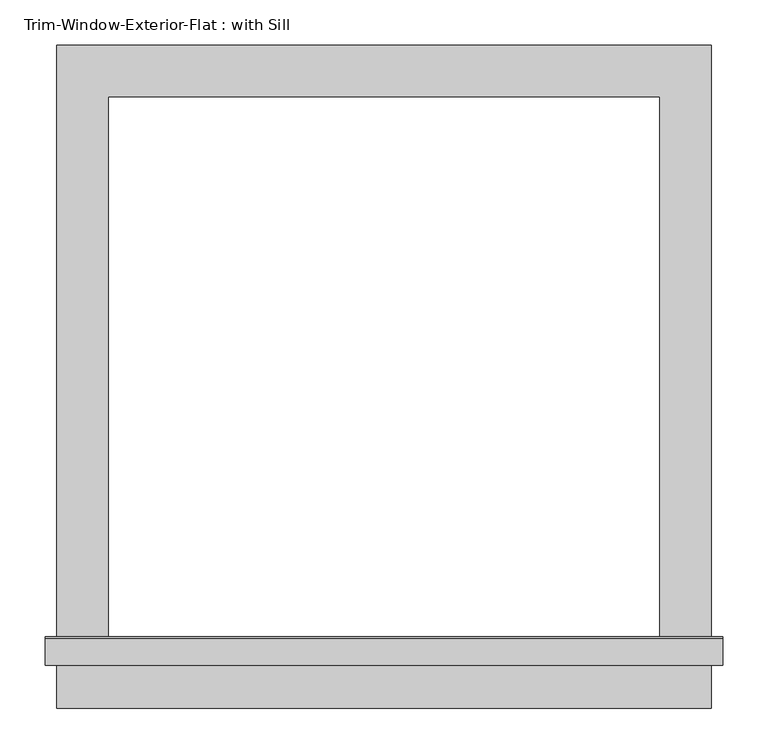
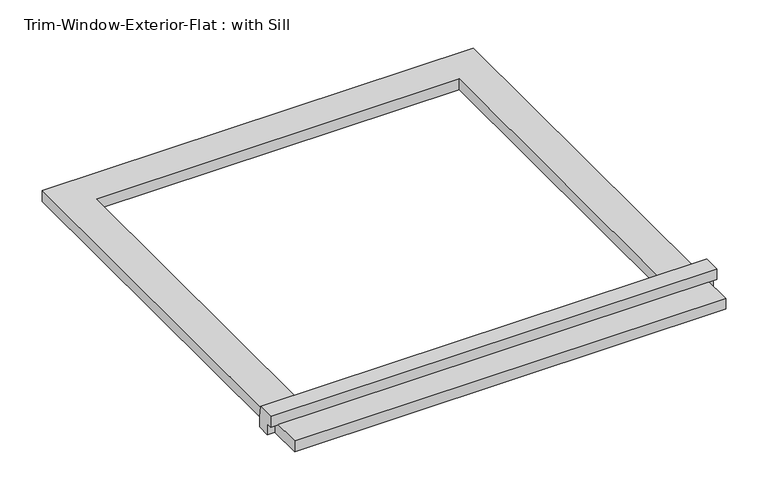
"""IFC4 building model written with IfcOpenShell, lengths in millimetres: proxy geometry, Trim-Window-Exterior-Flat : with Sill."""

from ifc_helpers import new_model, si_unit, frame, origin, origin_with_axes, place, context, project, spatial, polyline, outline, extrude, source, transform, mapped, element, save


def trim_window_exterior_flat_with_sill_79c463f4(model_context):
    return source(origin(), model_context, "Body", "SweptSolid", [
        extrude(outline(polyline([(361.95, -619.0823709), (361.95, -676.2323709), (-361.95, -676.2323709), (-361.95, -619.0823709), (361.95, -619.0823709)])), origin_with_axes(), (0.0, 0.0, 1.0), 19.05),
        extrude(outline(polyline([(-628.65, 38.1), (-599.3580645, 38.1), (-596.9, 19.05), (-596.9, 0.0), (-619.0823709, 0.0), (-619.0823709, 19.05), (-628.65, 19.05), (-628.65, 38.1)])), frame((-374.65, 0.0, 0.0), z_axis=(1.0, 0.0, 0.0), x_axis=(0.0, 1.0, 0.0)), (0.0, 0.0, 1.0), 749.3),
        extrude(outline(polyline([(-361.95, 57.15), (361.95, 57.15), (361.95, -596.9), (304.8, -596.9), (304.8, 0.0), (-304.8, 0.0), (-304.8, -596.9), (-361.95, -596.9), (-361.95, 57.15)])), origin_with_axes(), (0.0, 0.0, 1.0), 19.05),
    ])


if __name__ == "__main__":
    model = new_model("IFC4")
    model_context = context("Model", 3, world=origin())
    ifc_project = project(units=[si_unit("LENGTHUNIT", "METRE", prefix="MILLI")], contexts=[model_context])
    site = spatial("IfcSite", under=ifc_project)
    building = spatial("IfcBuilding", under=site)
    placement = place(None, origin())
    trim_window_exterior_flat_with_sill_shape = trim_window_exterior_flat_with_sill_79c463f4(model_context)
    element("IfcBuildingElementProxy", 1, Name="Trim-Window-Exterior-Flat : with Sill", ObjectType="Trim-Window-Exterior-Flat : with Sill", at=placement, inside=building, context=model_context, shape_type="MappedRepresentation", body=[
        mapped(trim_window_exterior_flat_with_sill_shape, transform((0.0, 0.0, 0.0), x_axis=(1.0, 0.0, 0.0), y_axis=(0.0, 1.0, 0.0), z_axis=(0.0, 0.0, 1.0))),
    ])
    save(model, "model.ifc")

# Revit data of these elements
# Type "Trim-Window-Exterior-Flat : with Sill"
#   Trim Width = 0' - 2 1/4"
#   Trim Thickness_Picture Frame = 0' - 1 1/4"
#   Trim Thickness_with Sill = 0' - 0 3/4"
#   Sill Thickness = 0' - 1 1/4"
#   Opening Width [instance default] = 2' - 0"
#   Opening Height [instance default] = 3' - 0"
#   Default Elevation = 4' - 0"
#   Sill = yes
#   Picture Frame = no
#   Trim Material [instance default] = none
# Element 1 (IfcBuildingElementProxy, "Trim-Window-Exterior-Flat : with Sill")
#   Opening Height = 1' - 11 1/2"
#   Trim Material = Clad - White
#   Materials on its faces: "Clad - White"
# Materials
#   "Clad - White": class "Wood", colour RGB 242 242 238, transparency 0, Cost = 0
